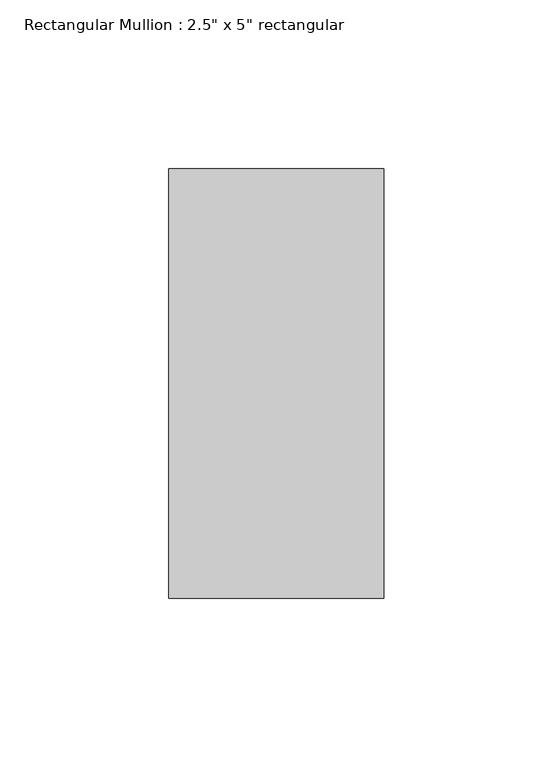
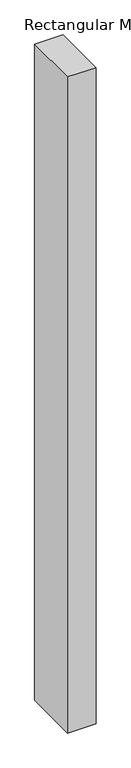
"""IFC4 building model written with IfcOpenShell, lengths in millimetres: member geometry."""

from ifc_helpers import new_model, si_unit, frame, origin, place, context, project, spatial, polyline, outline, extrude, source, transform, mapped, element, save


def member_fedd83b6(model_context):
    return source(origin(), model_context, "Body", "SweptSolid", [
        extrude(outline(polyline([(0.0, 63.5), (0.0, -63.5), (-63.5, -63.5), (-63.5, 63.5), (0.0, 63.5)])), frame((0.0, 0.0, -1549.4), z_axis=(0.0, 0.0, 1.0), x_axis=(1.0, 0.0, 0.0)), (0.0, 0.0, 1.0), 1549.4),
    ])


if __name__ == "__main__":
    model = new_model("IFC4")
    model_context = context("Model", 3, world=origin())
    ifc_project = project(units=[si_unit("LENGTHUNIT", "METRE", prefix="MILLI")], contexts=[model_context])
    site = spatial("IfcSite", under=ifc_project)
    building = spatial("IfcBuilding", under=site)
    placement = place(None, origin())
    member_shape = member_fedd83b6(model_context)
    element("IfcMember", 1, ObjectType="Rectangular Mullion : 2.5\" x 5\" rectangular", at=placement, inside=building, context=model_context, shape_type="MappedRepresentation", body=[
        mapped(member_shape, transform((0.0, 0.0, 0.0), x_axis=(1.0, 0.0, 0.0), y_axis=(0.0, 1.0, 0.0), z_axis=(0.0, 0.0, 1.0))),
    ])
    save(model, "model.ifc")

# Revit data of these elements
# Type "Rectangular Mullion : 2.5\" x 5\" rectangular"
#   built-in parameter 1007304 = 0.416667 (stored number, unit not read)
#   built-in parameter 1007301 = 0.104167 (stored number, unit not read)
#   built-in parameter 1007300 = 0.104167 (stored number, unit not read)
